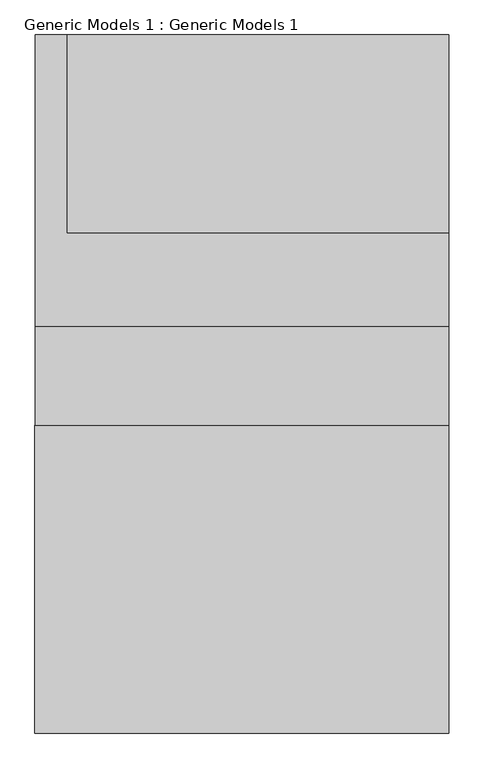
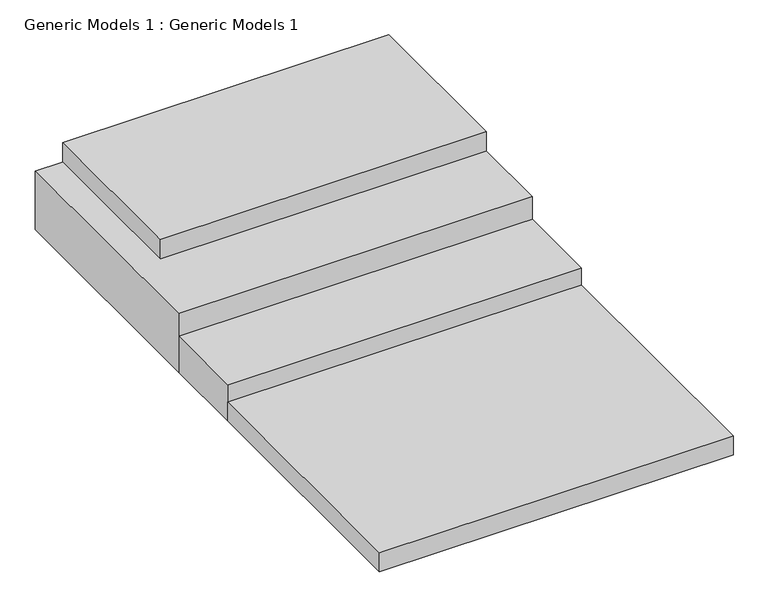
"""IFC4 building model written with IfcOpenShell, lengths in millimetres: proxy geometry, Generic Models 1 : Generic Models 1."""

from ifc_helpers import new_model, si_unit, frame, origin, place, context, project, spatial, polyline, outline, extrude, source, transform, mapped, element, save


def generic_models_1_generic_models_1_8db9de98(model_context):
    return source(origin(), model_context, "Body", "SweptSolid", [
        extrude(outline(polyline([(129.6588295, -7374.0266794), (129.6588295, -8639.3140259), (-2308.7411705, -8639.3140259), (-2308.7411705, -7374.0266794), (129.6588295, -7374.0266794)])), frame((0.0, 0.0, -616.5051112), z_axis=(0.0, 0.0, 1.0), x_axis=(1.0, 0.0, 0.0)), (0.0, 0.0, 1.0), 616.5051112),
        extrude(outline(polyline([(129.6588295, -8639.3140259), (129.6588295, -9236.0967491), (-2515.3370962, -9236.0967491), (-2515.3370962, -7374.0266794), (-2308.7411705, -7374.0266794), (-2308.7411705, -8639.3140259), (129.6588295, -8639.3140259)])), frame((0.0, 0.0, -616.5051112), z_axis=(0.0, 0.0, 1.0), x_axis=(1.0, 0.0, 0.0)), (0.0, 0.0, 1.0), 464.1051112),
        extrude(outline(polyline([(129.6588295, -9236.0967491), (129.6588295, -9870.9794723), (-2515.3370962, -9870.9794723), (-2515.3370962, -9236.0967491), (129.6588295, -9236.0967491)])), frame((0.0, 0.0, -616.5051112), z_axis=(0.0, 0.0, 1.0), x_axis=(1.0, 0.0, 0.0)), (0.0, 0.0, 1.0), 286.3051112),
        extrude(outline(polyline([(129.6588295, -11838.9642785), (-2516.4823872, -11838.9642785), (-2516.4823872, -9870.9794723), (129.6588295, -9870.9794723), (129.6588295, -11838.9642785)])), frame((0.0, 0.0, -616.5051112), z_axis=(0.0, 0.0, 1.0), x_axis=(1.0, 0.0, 0.0)), (0.0, 0.0, 1.0), 150.4160441),
    ])


if __name__ == "__main__":
    model = new_model("IFC4")
    model_context = context("Model", 3, world=origin())
    ifc_project = project(units=[si_unit("LENGTHUNIT", "METRE", prefix="MILLI")], contexts=[model_context])
    site = spatial("IfcSite", under=ifc_project)
    building = spatial("IfcBuilding", under=site)
    placement = place(None, origin())
    generic_models_1_generic_models_1_shape = generic_models_1_generic_models_1_8db9de98(model_context)
    element("IfcBuildingElementProxy", 1, Name="Generic Models 1 : Generic Models 1", ObjectType="Generic Models 1 : Generic Models 1", at=placement, inside=building, context=model_context, shape_type="MappedRepresentation", body=[
        mapped(generic_models_1_generic_models_1_shape, transform((0.0, 0.0, 0.0), x_axis=(1.0, 0.0, 0.0), y_axis=(0.0, 1.0, 0.0), z_axis=(0.0, 0.0, 1.0))),
    ])
    save(model, "model.ifc")
